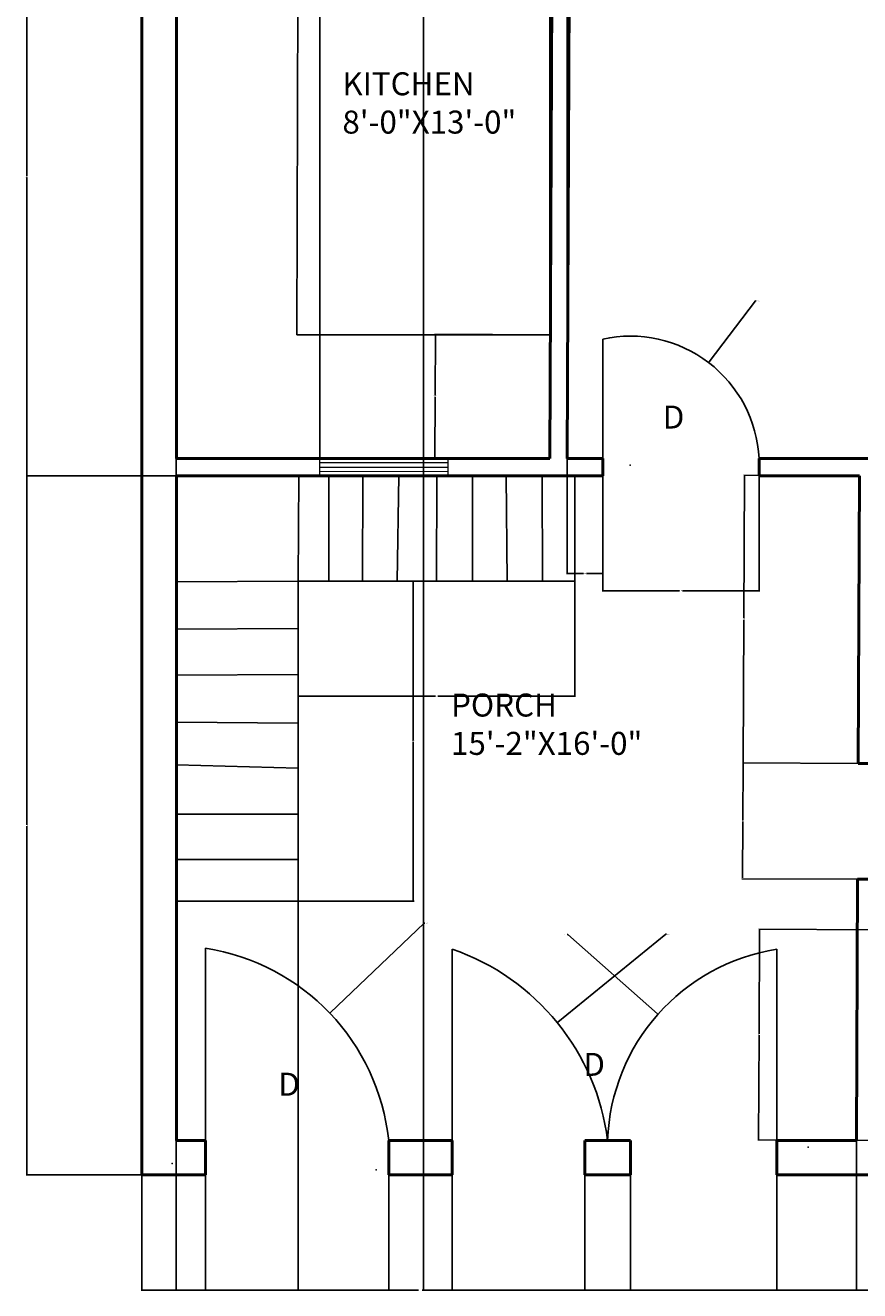
# Model space of a CAD drawing. Units: inches. Extents: x 2341 to 2761, y 2129 to 2789.
# Tile 1 of 4: x 2341 to 2559, y 2129 to 2459. Entities that reach past the tile are written whole.
import ezdxf

# ---------------------------------------------------------------- set-up
doc = ezdxf.new("R2010")
doc.units = ezdxf.units.IN
for name, color, linetype, lineweight in [('A-ANNO-DIMS', 2, 'Continuous', 18), ('A-ANNO-TEXT', 7, 'Continuous', 18), ('A-AREA-IDEN', 7, 'Continuous', 25), ('A-DOOR', 3, 'Continuous', 25), ('A-FLOR-FIXT', 9, 'Continuous', 25), ('A-FLOR-STRS', 7, 'Continuous', 25), ('A-GLAZ', 4, 'Continuous', 18), ('A-WALL', 7, 'Continuous', 50)]:
    doc.layers.add(name, color=color, linetype=linetype, lineweight=lineweight)
doc.styles.get("Standard").update_dxf_attribs({"font": 'arial.ttf'})
doc.dimstyles.get("Standard").update_dxf_attribs({"dimtxt": 0.18, "dimasz": 0.18, "dimexe": 0.18, "dimexo": 0.0625, "dimgap": 0.09, "dimtad": 0, "dimtih": 1, "dimtoh": 1, "dimdec": 4, "dimzin": 0, "dimdsep": 46, "dimtxsty": 'Standard', "dimcen": 0.09, "dimadec": 0, "dimazin": 0, "dimtfac": 1, "dimtdec": 4, "dimtofl": 0, "dimtmove": 0, "dimatfit": 3, "dimfxl": 1, "dimtolj": 1, "dimtzin": 0, "dimarcsym": 0})

# ---------------------------------------------------------------- blocks, each defined once
blk = doc.blocks.new('WIN-33IN-NARROW')
for p, q in [((0, 3.43), (33.34, 3.43)), ((0, 2.27), (33.34, 2.27)), ((0, 1.23), (33.34, 1.12))]:
    blk.add_line(p, q)
blk.add_lwpolyline([(0, 4.54), (33.34, 4.54), (33.34, 0), (0, 0)], close=True)
blk = doc.blocks.new('*D13')
at = {"layer": 'A-ANNO-DIMS', "color": 0, "lineweight": -2, "transparency": 16777216}
for p, q in [((2380.18, 2341.58), (2341.01, 2341.58)), ((2341.19, 2341.4), (2341.19, 2250.53)), ((2341.19, 2159.3), (2341.19, 2250.17)), ((2371.18, 2159.12), (2341.01, 2159.12))]:
    blk.add_line(p, q, dxfattribs=at)
at = {"layer": 'A-ANNO-DIMS', "color": 0, "transparency": 16777216}
for points in [[(2341.16, 2341.4), (2341.22, 2341.4), (2341.19, 2341.58)], [(2341.16, 2159.3), (2341.22, 2159.3), (2341.19, 2159.12)]]:
    blk.add_solid(points, dxfattribs=at)
at = {"layer": 'Defpoints', "color": 0, "transparency": 16777216}
for p in [(2341.19, 2341.58), (2380.24, 2341.58), (2371.24, 2159.12)]:
    blk.add_point(p, dxfattribs=at)
at = {"layer": 'A-ANNO-DIMS', "color": 0, "transparency": 16777216, "insert": (2341.19, 2250.35), "char_height": 0.18, "attachment_point": 5}
blk.add_mtext('\\A1;182.46', dxfattribs=at)
blk = doc.blocks.new('*D14')
at = {"layer": 'A-ANNO-DIMS', "color": 0, "lineweight": -2, "transparency": 16777216}
for p, q in [((2380.18, 2497.6), (2341.01, 2497.6)), ((2341.19, 2497.42), (2341.19, 2419.77)), ((2341.19, 2341.76), (2341.19, 2419.4)), ((2380.18, 2341.58), (2341.01, 2341.58))]:
    blk.add_line(p, q, dxfattribs=at)
at = {"layer": 'A-ANNO-DIMS', "color": 0, "transparency": 16777216}
for points in [[(2341.16, 2497.42), (2341.22, 2497.42), (2341.19, 2497.6)], [(2341.16, 2341.76), (2341.22, 2341.76), (2341.19, 2341.58)]]:
    blk.add_solid(points, dxfattribs=at)
at = {"layer": 'Defpoints', "color": 0, "transparency": 16777216}
for p in [(2341.19, 2497.6), (2380.24, 2497.6), (2380.24, 2341.58)]:
    blk.add_point(p, dxfattribs=at)
at = {"layer": 'A-ANNO-DIMS', "color": 0, "transparency": 16777216, "insert": (2341.19, 2419.59), "char_height": 0.18, "attachment_point": 5}
blk.add_mtext('\\A1;156.02', dxfattribs=at)
blk = doc.blocks.new('*D17')
at = {"layer": 'A-ANNO-DIMS', "color": 0, "lineweight": -2, "transparency": 16777216}
for p, q in [((2444.74, 2750.05), (2444.74, 2128.92)), ((2658.39, 2749.97), (2658.39, 2128.92)), ((2444.92, 2129.1), (2551.1, 2129.1)), ((2658.21, 2129.1), (2552.03, 2129.1))]:
    blk.add_line(p, q, dxfattribs=at)
at = {"layer": 'A-ANNO-DIMS', "color": 0, "transparency": 16777216}
for points in [[(2444.92, 2129.13), (2444.92, 2129.07), (2444.74, 2129.1)], [(2658.21, 2129.13), (2658.21, 2129.07), (2658.39, 2129.1)]]:
    blk.add_solid(points, dxfattribs=at)
at = {"layer": 'Defpoints', "color": 0, "transparency": 16777216}
for p in [(2444.74, 2750.12), (2658.39, 2750.04), (2658.39, 2129.1)]:
    blk.add_point(p, dxfattribs=at)
at = {"layer": 'A-ANNO-DIMS', "color": 0, "transparency": 16777216, "insert": (2551.56, 2129.1), "char_height": 0.18, "attachment_point": 5}
blk.add_mtext('\\A1;213.65', dxfattribs=at)
blk = doc.blocks.new('*D18')
at = {"layer": 'A-ANNO-DIMS', "color": 0, "lineweight": -2, "transparency": 16777216}
for p, q in [((2371.24, 2159.06), (2371.24, 2128.92)), ((2387.84, 2159.06), (2387.84, 2128.92)), ((2371.42, 2129.1), (2379.08, 2129.1)), ((2387.66, 2129.1), (2379.99, 2129.1))]:
    blk.add_line(p, q, dxfattribs=at)
at = {"layer": 'A-ANNO-DIMS', "color": 0, "transparency": 16777216}
for points in [[(2371.42, 2129.13), (2371.42, 2129.07), (2371.24, 2129.1)], [(2387.66, 2129.13), (2387.66, 2129.07), (2387.84, 2129.1)]]:
    blk.add_solid(points, dxfattribs=at)
at = {"layer": 'Defpoints', "color": 0, "transparency": 16777216}
for p in [(2371.24, 2159.12), (2387.84, 2159.12), (2387.84, 2129.1)]:
    blk.add_point(p, dxfattribs=at)
at = {"layer": 'A-ANNO-DIMS', "color": 0, "transparency": 16777216, "insert": (2379.54, 2129.1), "char_height": 0.18, "attachment_point": 5}
blk.add_mtext('\\A1;16.594', dxfattribs=at)
blk = doc.blocks.new('*D19')
at = {"layer": 'A-ANNO-DIMS', "color": 0, "lineweight": -2, "transparency": 16777216}
for p, q in [((2387.84, 2159.06), (2387.84, 2128.92)), ((2435.67, 2159.06), (2435.67, 2128.92)), ((2388.02, 2129.1), (2411.35, 2129.1)), ((2435.49, 2129.1), (2412.15, 2129.1))]:
    blk.add_line(p, q, dxfattribs=at)
at = {"layer": 'A-ANNO-DIMS', "color": 0, "transparency": 16777216}
for points in [[(2388.02, 2129.13), (2388.02, 2129.07), (2387.84, 2129.1)], [(2435.49, 2129.13), (2435.49, 2129.07), (2435.67, 2129.1)]]:
    blk.add_solid(points, dxfattribs=at)
at = {"layer": 'Defpoints', "color": 0, "transparency": 16777216}
for p in [(2387.84, 2159.12), (2435.67, 2159.12), (2435.67, 2129.1)]:
    blk.add_point(p, dxfattribs=at)
at = {"layer": 'A-ANNO-DIMS', "color": 0, "transparency": 16777216, "insert": (2411.75, 2129.1), "char_height": 0.18, "attachment_point": 5}
blk.add_mtext('\\A1;47.83', dxfattribs=at)
blk = doc.blocks.new('*D20')
at = {"layer": 'A-ANNO-DIMS', "color": 0, "lineweight": -2, "transparency": 16777216}
for p, q in [((2435.67, 2159.06), (2435.67, 2128.92)), ((2452.23, 2159.06), (2452.23, 2128.92)), ((2435.85, 2129.1), (2443.49, 2129.1)), ((2452.05, 2129.1), (2444.4, 2129.1))]:
    blk.add_line(p, q, dxfattribs=at)
at = {"layer": 'A-ANNO-DIMS', "color": 0, "transparency": 16777216}
for points in [[(2435.85, 2129.13), (2435.85, 2129.07), (2435.67, 2129.1)], [(2452.05, 2129.13), (2452.05, 2129.07), (2452.23, 2129.1)]]:
    blk.add_solid(points, dxfattribs=at)
at = {"layer": 'Defpoints', "color": 0, "transparency": 16777216}
for p in [(2435.67, 2159.12), (2452.23, 2159.12), (2452.23, 2129.1)]:
    blk.add_point(p, dxfattribs=at)
at = {"layer": 'A-ANNO-DIMS', "color": 0, "transparency": 16777216, "insert": (2443.95, 2129.1), "char_height": 0.18, "attachment_point": 5}
blk.add_mtext('\\A1;16.563', dxfattribs=at)
blk = doc.blocks.new('*D21')
at = {"layer": 'A-ANNO-DIMS', "color": 0, "lineweight": -2, "transparency": 16777216}
for p, q in [((2452.23, 2159.06), (2452.23, 2128.92)), ((2486.83, 2159.06), (2486.83, 2128.92)), ((2452.41, 2129.1), (2469.21, 2129.1)), ((2486.65, 2129.1), (2469.85, 2129.1))]:
    blk.add_line(p, q, dxfattribs=at)
at = {"layer": 'A-ANNO-DIMS', "color": 0, "transparency": 16777216}
for points in [[(2452.41, 2129.13), (2452.41, 2129.07), (2452.23, 2129.1)], [(2486.65, 2129.13), (2486.65, 2129.07), (2486.83, 2129.1)]]:
    blk.add_solid(points, dxfattribs=at)
at = {"layer": 'Defpoints', "color": 0, "transparency": 16777216}
for p in [(2452.23, 2159.12), (2486.83, 2159.12), (2486.83, 2129.1)]:
    blk.add_point(p, dxfattribs=at)
at = {"layer": 'A-ANNO-DIMS', "color": 0, "transparency": 16777216, "insert": (2469.53, 2129.1), "char_height": 0.18, "attachment_point": 5}
blk.add_mtext('\\A1;34.6', dxfattribs=at)
blk = doc.blocks.new('*D22')
at = {"layer": 'A-ANNO-DIMS', "color": 0, "lineweight": -2, "transparency": 16777216}
for p, q in [((2486.83, 2159.06), (2486.83, 2128.92)), ((2498.83, 2159.06), (2498.83, 2128.92)), ((2487.01, 2129.1), (2492.37, 2129.1)), ((2498.65, 2129.1), (2493.28, 2129.1))]:
    blk.add_line(p, q, dxfattribs=at)
at = {"layer": 'A-ANNO-DIMS', "color": 0, "transparency": 16777216}
for points in [[(2487.01, 2129.13), (2487.01, 2129.07), (2486.83, 2129.1)], [(2498.65, 2129.13), (2498.65, 2129.07), (2498.83, 2129.1)]]:
    blk.add_solid(points, dxfattribs=at)
at = {"layer": 'Defpoints', "color": 0, "transparency": 16777216}
for p in [(2486.83, 2159.12), (2498.83, 2159.12), (2498.83, 2129.1)]:
    blk.add_point(p, dxfattribs=at)
at = {"layer": 'A-ANNO-DIMS', "color": 0, "transparency": 16777216, "insert": (2492.83, 2129.1), "char_height": 0.18, "attachment_point": 5}
blk.add_mtext('\\A1;11.996', dxfattribs=at)
blk = doc.blocks.new('*D23')
at = {"layer": 'A-ANNO-DIMS', "color": 0, "lineweight": -2, "transparency": 16777216}
for p, q in [((2498.83, 2159.06), (2498.83, 2128.92)), ((2537.01, 2159.06), (2537.01, 2128.92)), ((2499.01, 2129.1), (2517.52, 2129.1)), ((2536.83, 2129.1), (2518.31, 2129.1))]:
    blk.add_line(p, q, dxfattribs=at)
at = {"layer": 'A-ANNO-DIMS', "color": 0, "transparency": 16777216}
for points in [[(2499.01, 2129.13), (2499.01, 2129.07), (2498.83, 2129.1)], [(2536.83, 2129.13), (2536.83, 2129.07), (2537.01, 2129.1)]]:
    blk.add_solid(points, dxfattribs=at)
at = {"layer": 'Defpoints', "color": 0, "transparency": 16777216}
for p in [(2498.83, 2159.12), (2537.01, 2159.12), (2537.01, 2129.1)]:
    blk.add_point(p, dxfattribs=at)
at = {"layer": 'A-ANNO-DIMS', "color": 0, "transparency": 16777216, "insert": (2517.92, 2129.1), "char_height": 0.18, "attachment_point": 5}
blk.add_mtext('\\A1;38.18', dxfattribs=at)
blk = doc.blocks.new('*D24')
at = {"layer": 'A-ANNO-DIMS', "color": 0, "lineweight": -2, "transparency": 16777216}
for p, q in [((2557.74, 2168.07), (2557.74, 2128.92)), ((2537.01, 2159.06), (2537.01, 2128.92)), ((2537.19, 2129.1), (2546.91, 2129.1)), ((2557.56, 2129.1), (2547.84, 2129.1))]:
    blk.add_line(p, q, dxfattribs=at)
at = {"layer": 'A-ANNO-DIMS', "color": 0, "transparency": 16777216}
for points in [[(2537.19, 2129.13), (2537.19, 2129.07), (2537.01, 2129.1)], [(2557.56, 2129.13), (2557.56, 2129.07), (2557.74, 2129.1)]]:
    blk.add_solid(points, dxfattribs=at)
at = {"layer": 'Defpoints', "color": 0, "transparency": 16777216}
for p in [(2557.74, 2168.13), (2537.01, 2159.12), (2557.74, 2129.1)]:
    blk.add_point(p, dxfattribs=at)
at = {"layer": 'A-ANNO-DIMS', "color": 0, "transparency": 16777216, "insert": (2547.37, 2129.1), "char_height": 0.18, "attachment_point": 5}
blk.add_mtext('\\A1;20.736', dxfattribs=at)
blk = doc.blocks.new('*D25')
at = {"layer": 'A-ANNO-DIMS', "color": 0, "lineweight": -2, "transparency": 16777216}
for p, q in [((2557.74, 2168.07), (2557.74, 2128.92)), ((2650.24, 2168.1), (2650.24, 2128.92)), ((2557.92, 2129.1), (2603.67, 2129.1)), ((2650.06, 2129.1), (2604.32, 2129.1))]:
    blk.add_line(p, q, dxfattribs=at)
at = {"layer": 'A-ANNO-DIMS', "color": 0, "transparency": 16777216}
for points in [[(2557.92, 2129.13), (2557.92, 2129.07), (2557.74, 2129.1)], [(2650.06, 2129.13), (2650.06, 2129.07), (2650.24, 2129.1)]]:
    blk.add_solid(points, dxfattribs=at)
at = {"layer": 'Defpoints', "color": 0, "transparency": 16777216}
for p in [(2557.74, 2168.13), (2650.24, 2168.16), (2650.24, 2129.1)]:
    blk.add_point(p, dxfattribs=at)
at = {"layer": 'A-ANNO-DIMS', "color": 0, "transparency": 16777216, "insert": (2603.99, 2129.1), "char_height": 0.18, "attachment_point": 5}
blk.add_mtext('\\A1;92.5', dxfattribs=at)
blk = doc.blocks.new('*D27')
at = {"layer": 'A-ANNO-DIMS', "color": 0, "lineweight": -2, "transparency": 16777216}
for p, q in [((2380.24, 2230.49), (2380.24, 2128.92)), ((2412.08, 2230.49), (2412.08, 2128.92)), ((2380.42, 2129.1), (2395.77, 2129.1)), ((2411.9, 2129.1), (2396.56, 2129.1))]:
    blk.add_line(p, q, dxfattribs=at)
at = {"layer": 'A-ANNO-DIMS', "color": 0, "transparency": 16777216}
for points in [[(2380.42, 2129.13), (2380.42, 2129.07), (2380.24, 2129.1)], [(2411.9, 2129.13), (2411.9, 2129.07), (2412.08, 2129.1)]]:
    blk.add_solid(points, dxfattribs=at)
at = {"layer": 'Defpoints', "color": 0, "transparency": 16777216}
for p in [(2380.24, 2230.56), (2412.08, 2230.56), (2412.08, 2129.1)]:
    blk.add_point(p, dxfattribs=at)
at = {"layer": 'A-ANNO-DIMS', "color": 0, "transparency": 16777216, "insert": (2396.16, 2129.1), "char_height": 0.18, "attachment_point": 5}
blk.add_mtext('\\A1;31.84', dxfattribs=at)
blk = doc.blocks.new('*D28')
at = {"layer": 'A-ANNO-DIMS', "color": 0, "lineweight": -2, "transparency": 16777216}
for p, q in [((2477.74, 2346.18), (2477.74, 2789.36)), ((2477.92, 2789.18), (2479.73, 2789.18)), ((2482.06, 2789.18), (2480.25, 2789.18)), ((2482.24, 2346.16), (2482.24, 2789.36))]:
    blk.add_line(p, q, dxfattribs=at)
at = {"layer": 'A-ANNO-DIMS', "color": 0, "transparency": 16777216}
for points in [[(2477.92, 2789.21), (2477.92, 2789.15), (2477.74, 2789.18)], [(2482.06, 2789.21), (2482.06, 2789.15), (2482.24, 2789.18)]]:
    blk.add_solid(points, dxfattribs=at)
at = {"layer": 'Defpoints', "color": 0, "transparency": 16777216}
for p in [(2482.24, 2789.18), (2477.74, 2346.12), (2482.24, 2346.1)]:
    blk.add_point(p, dxfattribs=at)
at = {"layer": 'A-ANNO-DIMS', "color": 0, "transparency": 16777216, "insert": (2479.99, 2789.18), "char_height": 0.18, "attachment_point": 5}
blk.add_mtext('\\A1;4.5', dxfattribs=at)
blk = doc.blocks.new('*D29')
at = {"layer": 'A-ANNO-DIMS', "color": 0, "lineweight": -2, "transparency": 16777216}
for p, q in [((2371.24, 2759.06), (2371.24, 2128.92)), ((2380.24, 2750.06), (2380.24, 2128.92)), ((2371.42, 2129.1), (2375.59, 2129.1)), ((2380.06, 2129.1), (2375.89, 2129.1))]:
    blk.add_line(p, q, dxfattribs=at)
at = {"layer": 'A-ANNO-DIMS', "color": 0, "transparency": 16777216}
for points in [[(2371.42, 2129.13), (2371.42, 2129.07), (2371.24, 2129.1)], [(2380.06, 2129.13), (2380.06, 2129.07), (2380.24, 2129.1)]]:
    blk.add_solid(points, dxfattribs=at)
at = {"layer": 'Defpoints', "color": 0, "transparency": 16777216}
for p in [(2371.24, 2759.12), (2380.24, 2750.12), (2380.24, 2129.1)]:
    blk.add_point(p, dxfattribs=at)
at = {"layer": 'A-ANNO-DIMS', "color": 0, "transparency": 16777216, "insert": (2375.74, 2129.1), "char_height": 0.18, "attachment_point": 5}
blk.add_mtext('\\A1;9', dxfattribs=at)
blk = doc.blocks.new('*D30')
at = {"layer": 'A-ANNO-DIMS', "color": 0, "lineweight": -2, "transparency": 16777216}
for p, q in [((2562.45, 2223.1), (2532.31, 2223.25)), ((2532.49, 2223.06), (2532.36, 2195.94)), ((2532.22, 2168.45), (2532.36, 2195.58)), ((2562.18, 2168.12), (2532.04, 2168.27))]:
    blk.add_line(p, q, dxfattribs=at)
at = {"layer": 'A-ANNO-DIMS', "color": 0, "transparency": 16777216}
for points in [[(2532.46, 2223.06), (2532.52, 2223.06), (2532.49, 2223.24)], [(2532.19, 2168.45), (2532.25, 2168.45), (2532.22, 2168.27)]]:
    blk.add_solid(points, dxfattribs=at)
at = {"layer": 'Defpoints', "color": 0, "transparency": 16777216}
for p in [(2532.49, 2223.24), (2562.51, 2223.1), (2562.24, 2168.12)]:
    blk.add_point(p, dxfattribs=at)
at = {"layer": 'A-ANNO-DIMS', "color": 0, "transparency": 16777216, "insert": (2532.36, 2195.76), "char_height": 0.18, "attachment_point": 5}
blk.add_mtext('\\A1;54.97', dxfattribs=at)
blk = doc.blocks.new('*D33')
at = {"layer": 'A-ANNO-DIMS', "color": 0, "lineweight": -2, "transparency": 16777216}
for p, q in [((2380.24, 2346.14), (2380.24, 2789.36)), ((2380.42, 2789.18), (2398.59, 2789.18)), ((2417.55, 2789.18), (2399.38, 2789.18)), ((2417.73, 2346.19), (2417.73, 2789.36))]:
    blk.add_line(p, q, dxfattribs=at)
at = {"layer": 'A-ANNO-DIMS', "color": 0, "transparency": 16777216}
for points in [[(2380.42, 2789.21), (2380.42, 2789.15), (2380.24, 2789.18)], [(2417.55, 2789.21), (2417.55, 2789.15), (2417.73, 2789.18)]]:
    blk.add_solid(points, dxfattribs=at)
at = {"layer": 'Defpoints', "color": 0, "transparency": 16777216}
for p in [(2417.73, 2789.18), (2380.24, 2346.08), (2417.73, 2346.13)]:
    blk.add_point(p, dxfattribs=at)
at = {"layer": 'A-ANNO-DIMS', "color": 0, "transparency": 16777216, "insert": (2398.99, 2789.18), "char_height": 0.18, "attachment_point": 5}
blk.add_mtext('\\A1;37.49', dxfattribs=at)
blk = doc.blocks.new('*D49')
at = {"layer": 'A-ANNO-DIMS', "color": 0, "lineweight": -2, "transparency": 16777216}
for p, q in [((2482.24, 2346.03), (2482.24, 2315.9)), ((2491.53, 2346.03), (2491.53, 2315.9)), ((2482.42, 2316.08), (2486.49, 2316.08)), ((2491.35, 2316.08), (2487.28, 2316.08))]:
    blk.add_line(p, q, dxfattribs=at)
at = {"layer": 'A-ANNO-DIMS', "color": 0, "transparency": 16777216}
for points in [[(2482.42, 2316.11), (2482.42, 2316.05), (2482.24, 2316.08)], [(2491.35, 2316.11), (2491.35, 2316.05), (2491.53, 2316.08)]]:
    blk.add_solid(points, dxfattribs=at)
at = {"layer": 'Defpoints', "color": 0, "transparency": 16777216}
for p in [(2482.24, 2346.1), (2491.53, 2346.1), (2482.24, 2316.08)]:
    blk.add_point(p, dxfattribs=at)
at = {"layer": 'A-ANNO-DIMS', "color": 0, "transparency": 16777216, "insert": (2486.89, 2316.08), "char_height": 0.18, "attachment_point": 5}
blk.add_mtext('\\A1;9.296', dxfattribs=at)
blk = doc.blocks.new('*D50')
at = {"layer": 'A-ANNO-DIMS', "color": 0, "lineweight": -2, "transparency": 16777216}
for p, q in [((2491.53, 2341.53), (2491.53, 2311.4)), ((2532.36, 2341.53), (2532.36, 2311.4)), ((2491.71, 2311.58), (2511.55, 2311.58)), ((2532.18, 2311.58), (2512.34, 2311.58))]:
    blk.add_line(p, q, dxfattribs=at)
at = {"layer": 'A-ANNO-DIMS', "color": 0, "transparency": 16777216}
for points in [[(2491.71, 2311.61), (2491.71, 2311.55), (2491.53, 2311.58)], [(2532.18, 2311.61), (2532.18, 2311.55), (2532.36, 2311.58)]]:
    blk.add_solid(points, dxfattribs=at)
at = {"layer": 'Defpoints', "color": 0, "transparency": 16777216}
for p in [(2491.53, 2341.6), (2532.36, 2341.6), (2491.53, 2311.58)]:
    blk.add_point(p, dxfattribs=at)
at = {"layer": 'A-ANNO-DIMS', "color": 0, "transparency": 16777216, "insert": (2511.95, 2311.58), "char_height": 0.18, "attachment_point": 5}
blk.add_mtext('\\A1;40.82', dxfattribs=at)
blk = doc.blocks.new('*D51')
at = {"layer": 'A-ANNO-DIMS', "color": 0, "lineweight": -2, "transparency": 16777216}
for p, q in [((2558.17, 2266.54), (2528.03, 2266.69)), ((2528.21, 2266.51), (2528.14, 2251.75)), ((2528.06, 2236.62), (2528.13, 2251.38)), ((2558.02, 2236.29), (2527.88, 2236.44))]:
    blk.add_line(p, q, dxfattribs=at)
at = {"layer": 'A-ANNO-DIMS', "color": 0, "transparency": 16777216}
for points in [[(2528.18, 2266.51), (2528.24, 2266.51), (2528.21, 2266.69)], [(2528.03, 2236.62), (2528.09, 2236.62), (2528.06, 2236.44)]]:
    blk.add_solid(points, dxfattribs=at)
at = {"layer": 'Defpoints', "color": 0, "transparency": 16777216}
for p in [(2528.21, 2266.69), (2558.23, 2266.54), (2558.08, 2236.29)]:
    blk.add_point(p, dxfattribs=at)
at = {"layer": 'A-ANNO-DIMS', "color": 0, "transparency": 16777216, "insert": (2528.14, 2251.56), "char_height": 0.18, "attachment_point": 5}
blk.add_mtext('\\A1;30.25', dxfattribs=at)
blk = doc.blocks.new('*D52')
at = {"layer": 'A-ANNO-DIMS', "color": 0, "lineweight": -2, "transparency": 16777216}
for p, q in [((2558.54, 2341.6), (2528.4, 2341.75)), ((2528.58, 2341.56), (2528.4, 2304.4)), ((2528.21, 2266.87), (2528.4, 2304.03)), ((2558.17, 2266.54), (2528.03, 2266.69))]:
    blk.add_line(p, q, dxfattribs=at)
at = {"layer": 'A-ANNO-DIMS', "color": 0, "transparency": 16777216}
for points in [[(2528.55, 2341.56), (2528.61, 2341.56), (2528.58, 2341.74)], [(2528.18, 2266.87), (2528.24, 2266.87), (2528.21, 2266.69)]]:
    blk.add_solid(points, dxfattribs=at)
at = {"layer": 'Defpoints', "color": 0, "transparency": 16777216}
for p in [(2528.58, 2341.74), (2558.6, 2341.6), (2558.23, 2266.54)]:
    blk.add_point(p, dxfattribs=at)
at = {"layer": 'A-ANNO-DIMS', "color": 0, "transparency": 16777216, "insert": (2528.4, 2304.22), "char_height": 0.18, "attachment_point": 5}
blk.add_mtext('\\A1;75.06', dxfattribs=at)
blk = doc.blocks.new('*D56')
at = {"layer": 'A-ANNO-DIMS', "color": 0, "lineweight": -2, "transparency": 16777216}
for p, q in [((2412.15, 2314.12), (2442.28, 2314.12)), ((2442.1, 2313.94), (2442.1, 2272.52)), ((2442.1, 2230.74), (2442.1, 2272.16)), ((2412.15, 2230.56), (2442.28, 2230.56))]:
    blk.add_line(p, q, dxfattribs=at)
at = {"layer": 'A-ANNO-DIMS', "color": 0, "transparency": 16777216}
for points in [[(2442.07, 2313.94), (2442.13, 2313.94), (2442.1, 2314.12)], [(2442.07, 2230.74), (2442.13, 2230.74), (2442.1, 2230.56)]]:
    blk.add_solid(points, dxfattribs=at)
at = {"layer": 'Defpoints', "color": 0, "transparency": 16777216}
for p in [(2412.08, 2314.12), (2412.08, 2230.56), (2442.1, 2230.56)]:
    blk.add_point(p, dxfattribs=at)
at = {"layer": 'A-ANNO-DIMS', "color": 0, "transparency": 16777216, "insert": (2442.1, 2272.34), "char_height": 0.18, "attachment_point": 5}
blk.add_mtext('\\A1;83.57', dxfattribs=at)
blk = doc.blocks.new('*D57')
at = {"layer": 'A-ANNO-DIMS', "color": 0, "lineweight": -2, "transparency": 16777216}
for p, q in [((2412.08, 2314.06), (2412.08, 2283.92)), ((2484.28, 2314.06), (2484.28, 2283.92)), ((2412.26, 2284.1), (2447.86, 2284.1)), ((2484.1, 2284.1), (2448.5, 2284.1))]:
    blk.add_line(p, q, dxfattribs=at)
at = {"layer": 'A-ANNO-DIMS', "color": 0, "transparency": 16777216}
for points in [[(2412.26, 2284.13), (2412.26, 2284.07), (2412.08, 2284.1)], [(2484.1, 2284.13), (2484.1, 2284.07), (2484.28, 2284.1)]]:
    blk.add_solid(points, dxfattribs=at)
at = {"layer": 'Defpoints', "color": 0, "transparency": 16777216}
for p in [(2412.08, 2314.12), (2484.28, 2314.12), (2412.08, 2284.1)]:
    blk.add_point(p, dxfattribs=at)
at = {"layer": 'A-ANNO-DIMS', "color": 0, "transparency": 16777216, "insert": (2448.18, 2284.1), "char_height": 0.18, "attachment_point": 5}
blk.add_mtext('\\A1;72.2', dxfattribs=at)
blk = doc.blocks.new('*D59')
at = {"layer": 'A-ANNO-DIMS', "color": 0, "lineweight": -2, "transparency": 16777216}
for p, q in [((2477.82, 2378.38), (2447.68, 2378.51)), ((2447.86, 2378.33), (2447.79, 2362.56)), ((2447.72, 2346.43), (2447.79, 2362.2)), ((2477.68, 2346.12), (2447.54, 2346.25))]:
    blk.add_line(p, q, dxfattribs=at)
at = {"layer": 'A-ANNO-DIMS', "color": 0, "transparency": 16777216}
for points in [[(2447.83, 2378.33), (2447.89, 2378.33), (2447.86, 2378.51)], [(2447.69, 2346.43), (2447.75, 2346.43), (2447.72, 2346.25)]]:
    blk.add_solid(points, dxfattribs=at)
at = {"layer": 'Defpoints', "color": 0, "transparency": 16777216}
for p in [(2447.86, 2378.51), (2477.88, 2378.38), (2477.74, 2346.12)]:
    blk.add_point(p, dxfattribs=at)
at = {"layer": 'A-ANNO-DIMS', "color": 0, "transparency": 16777216, "insert": (2447.79, 2362.38), "char_height": 0.18, "attachment_point": 5}
blk.add_mtext('\\A1;32.265', dxfattribs=at)
blk = doc.blocks.new('*D62')
at = {"layer": 'A-ANNO-DIMS', "color": 0, "lineweight": -2, "transparency": 16777216}
for p, q in [((2508.03, 2221.95), (2479.79, 2199)), ((2508.21, 2221.95), (2508.03, 2221.95)), ((2432.28, 2160.44), (2432.46, 2160.44)), ((2432.37, 2160.35), (2432.37, 2160.53))]:
    blk.add_line(p, q, dxfattribs=at)
at = {"layer": 'A-ANNO-DIMS', "color": 0, "transparency": 16777216}
blk.add_solid([(2479.78, 2199.02), (2479.81, 2198.98), (2479.66, 2198.89)], dxfattribs=at)
at = {"layer": 'Defpoints', "color": 0, "transparency": 16777216}
for p in [(2479.66, 2198.89), (2432.37, 2160.44)]:
    blk.add_point(p, dxfattribs=at)
at = {"layer": 'A-ANNO-DIMS', "color": 0, "transparency": 16777216, "insert": (2508.69, 2221.95), "char_height": 0.18, "attachment_point": 5}
blk.add_mtext('\\A1;R60.94', dxfattribs=at)
blk = doc.blocks.new('*D63')
at = {"layer": 'A-ANNO-DIMS', "color": 0, "lineweight": -2, "transparency": 16777216}
for p, q in [((2444.95, 2224.86), (2420.42, 2201.47)), ((2445.13, 2224.86), (2444.95, 2224.86)), ((2379.1, 2162.15), (2379.28, 2162.15)), ((2379.19, 2162.06), (2379.19, 2162.24))]:
    blk.add_line(p, q, dxfattribs=at)
at = {"layer": 'A-ANNO-DIMS', "color": 0, "transparency": 16777216}
blk.add_solid([(2420.4, 2201.49), (2420.44, 2201.45), (2420.29, 2201.34)], dxfattribs=at)
at = {"layer": 'Defpoints', "color": 0, "transparency": 16777216}
for p in [(2420.29, 2201.34), (2379.19, 2162.15)]:
    blk.add_point(p, dxfattribs=at)
at = {"layer": 'A-ANNO-DIMS', "color": 0, "transparency": 16777216, "insert": (2445.61, 2224.86), "char_height": 0.18, "attachment_point": 5}
blk.add_mtext('\\A1;R56.79', dxfattribs=at)
blk = doc.blocks.new('*D64')
at = {"layer": 'A-ANNO-DIMS', "color": 0, "lineweight": -2, "transparency": 16777216}
for p, q in [((2482.24, 2221.84), (2482.42, 2221.84)), ((2482.42, 2221.84), (2505.8, 2201.16)), ((2545.04, 2166.36), (2545.22, 2166.36)), ((2545.13, 2166.27), (2545.13, 2166.45))]:
    blk.add_line(p, q, dxfattribs=at)
at = {"layer": 'A-ANNO-DIMS', "color": 0, "transparency": 16777216}
blk.add_solid([(2505.82, 2201.18), (2505.78, 2201.13), (2505.94, 2201.04)], dxfattribs=at)
at = {"layer": 'Defpoints', "color": 0, "transparency": 16777216}
for p in [(2505.94, 2201.04), (2545.13, 2166.36)]:
    blk.add_point(p, dxfattribs=at)
at = {"layer": 'A-ANNO-DIMS', "color": 0, "transparency": 16777216, "insert": (2481.76, 2221.84), "char_height": 0.18, "attachment_point": 5}
blk.add_mtext('\\A1;R52.33', dxfattribs=at)
blk = doc.blocks.new('*D70')
at = {"layer": 'A-ANNO-DIMS', "color": 0, "lineweight": -2, "transparency": 16777216}
for p, q in [((2531.43, 2387.2), (2519.28, 2371.28)), ((2531.61, 2387.2), (2531.43, 2387.2)), ((2498.63, 2344.38), (2498.81, 2344.38)), ((2498.72, 2344.29), (2498.72, 2344.47))]:
    blk.add_line(p, q, dxfattribs=at)
at = {"layer": 'A-ANNO-DIMS', "color": 0, "transparency": 16777216}
blk.add_solid([(2519.25, 2371.3), (2519.3, 2371.26), (2519.17, 2371.14)], dxfattribs=at)
at = {"layer": 'Defpoints', "color": 0, "transparency": 16777216}
for p in [(2519.17, 2371.14), (2498.72, 2344.38)]:
    blk.add_point(p, dxfattribs=at)
at = {"layer": 'A-ANNO-DIMS', "color": 0, "transparency": 16777216, "insert": (2532.16, 2387.2), "char_height": 0.18, "attachment_point": 5}
blk.add_mtext('\\A1;R33.677', dxfattribs=at)

msp = doc.modelspace()

# ---------------------------------------------------------------- linework, layer by layer
at = {"layer": 'A-DOOR'}
for p, q in [((2491.5341, 2346.0958), (2491.5341, 2377.2773)), ((2387.8363, 2168.1222), (2387.8363, 2218.2792)), ((2452.2283, 2168.1247), (2452.2283, 2218.0539)), ((2537.0059, 2168.128), (2537.0057, 2218.0539))]:
    msp.add_line(p, q, dxfattribs=at)
for centre, radius, start, end in [((2498.7241, 2344.3772), 33.6765, 2.925153, 102.327529), ((2379.1921, 2162.1527), 56.7882, 6.035859, 81.244458), ((2432.3705, 2160.4354), 60.9444, 7.249744, 70.983867), ((2545.1263, 2166.3593), 52.3286, 98.927508, 178.064871)]:
    msp.add_arc(centre, radius, start, end, dxfattribs=at)
at = {"layer": 'A-FLOR-FIXT'}
for p, q in [((2411.7316, 2378.3809), (2412.0874, 2497.5958)), ((2477.8811, 2378.3809), (2411.7316, 2378.3809))]:
    msp.add_line(p, q, dxfattribs=at)
at = {"layer": 'A-FLOR-STRS'}
for p, q in [((2412.0845, 2314.1234), (2412.2571, 2341.5831)), ((2420.0237, 2314.1234), (2420.0236, 2341.5845)), ((2428.8188, 2314.1234), (2428.9607, 2341.5861)), ((2437.8824, 2314.1234), (2438.3072, 2341.5878)), ((2448.1827, 2314.1234), (2448.2205, 2341.5896)), ((2457.5672, 2314.1234), (2457.5672, 2341.5913)), ((2466.6307, 2314.1234), (2466.3475, 2341.5929)), ((2475.8359, 2314.1234), (2475.6942, 2341.5946)), ((2484.281, 2314.1234), (2484.281, 2341.5958)), ((2412.0845, 2314.1234), (2380.242, 2313.8851)), ((2412.0845, 2230.5563), (2412.0845, 2314.1234)), ((2412.0845, 2314.1234), (2484.281, 2314.1234)), ((2412.0845, 2301.7549), (2380.242, 2301.5284)), ((2412.0845, 2289.7474), (2380.242, 2289.5209)), ((2412.0845, 2277.0603), (2380.242, 2277.2869)), ((2412.0845, 2265.2794), (2380.242, 2266.1856)), ((2412.0845, 2253.2719), (2380.242, 2253.2719)), ((2412.0845, 2241.491), (2380.242, 2241.491)), ((2380.242, 2230.5563), (2412.0845, 2230.5563))]:
    msp.add_line(p, q, dxfattribs=at)
at = {"layer": 'A-WALL'}
for p, q in [((2371.242, 2159.1219), (2371.242, 2759.1219)), ((2380.242, 2346.0773), (2380.242, 2497.5958)), ((2477.7379, 2346.1158), (2478.3031, 2473.4534)), ((2482.2379, 2346.0958), (2482.8032, 2473.4534)), ((2380.242, 2346.0773), (2477.7379, 2346.1158)), ((2491.5341, 2346.0958), (2482.2379, 2346.0958)), ((2491.5341, 2346.0958), (2491.5341, 2341.5958)), ((2722.2379, 2346.0958), (2532.3567, 2346.0958)), ((2532.3567, 2346.0958), (2532.3567, 2341.5958)), ((2482.2387, 2341.5958), (2380.242, 2341.5773)), ((2380.242, 2168.1219), (2380.242, 2341.5773)), ((2491.5341, 2341.5958), (2482.2379, 2341.5958)), ((2558.6015, 2341.5958), (2532.3567, 2341.5958)), ((2558.2296, 2266.54), (2558.6015, 2341.5958)), ((2558.2296, 2266.54), (2562.7297, 2266.54)), ((2557.7421, 2168.1288), (2558.0798, 2236.2899)), ((2558.0798, 2236.2899), (2562.5798, 2236.2899)), ((2380.242, 2168.1219), (2387.8363, 2168.1222)), ((2387.8363, 2168.1222), (2387.8363, 2159.1219)), ((2435.6655, 2168.1241), (2452.2283, 2168.1247)), ((2435.6655, 2168.1241), (2435.6655, 2159.1219)), ((2452.2283, 2168.1247), (2452.2283, 2159.1219)), ((2486.8294, 2168.1261), (2498.8259, 2168.1265)), ((2486.8294, 2168.1261), (2486.8294, 2159.1219)), ((2498.8259, 2168.1265), (2498.8259, 2159.1219)), ((2537.0059, 2168.128), (2557.7421, 2168.1288)), ((2537.0059, 2168.128), (2537.006, 2159.1219)), ((2387.8363, 2159.1219), (2371.242, 2159.1219)), ((2452.2283, 2159.1219), (2435.6655, 2159.1219)), ((2498.8259, 2159.1219), (2486.8294, 2159.1219)), ((2731.242, 2159.1219), (2537.006, 2159.1219))]:
    msp.add_line(p, q, dxfattribs=at)

# ---------------------------------------------------------------- block references
at = {"layer": 'A-GLAZ'}
msp.add_blockref('WIN-33IN-NARROW', (2417.7311, 2341.5842), dxfattribs=at)

# ---------------------------------------------------------------- texts
at = {"layer": 'A-ANNO-TEXT', "char_height": 6, "attachment_point": 1}
for insert in [(2507.2133, 2359.9074), (2486.4801, 2190.9776), (2406.8635, 2185.8064)]:
    msp.add_mtext_dynamic_manual_height_columns('D', width=9.002909, gutter_width=12.5, heights=[0], dxfattribs=dict(at, insert=insert))
at = {"layer": 'A-AREA-IDEN', "char_height": 6, "attachment_point": 1}
for s, width, insert in [('KITCHEN \\P8\'-0"X13\'-0"', 36.809608, (2423.5911, 2446.8818)), ('PORCH\\P15\'-2"X16\'-0"', 72.299204, (2451.9445, 2284.7541))]:
    msp.add_mtext_dynamic_manual_height_columns(s, width=width, gutter_width=12.5, heights=[0], dxfattribs=dict(at, insert=insert))

# ---------------------------------------------------------------- dimensions: what is measured, and where the dimension line sits
at = {"layer": 'A-ANNO-DIMS'}
for base, p1, p2, override, picture, middle in [((2417.7307, 2789.1821), (2380.242, 2346.0773), (2417.7307, 2346.1252), {"dimdec": 2, "dimlfac": 1, "dimrnd": 0, "dimzin": 0, "dimdsep": 46, "dimlunit": 2}, '*D33', (2398.9864, 2789.1821)), ((2482.2379, 2789.1821), (2477.7379, 2346.1158), (2482.2379, 2346.0958), {"dimdec": 1, "dimlfac": 1, "dimrnd": 0, "dimzin": 0, "dimdsep": 46, "dimlunit": 2}, '*D28', (2479.9879, 2789.1821)), ((2380.242, 2129.1019), (2371.242, 2759.1219), (2380.242, 2750.1219), {"dimdec": 0, "dimlfac": 1, "dimrnd": 0, "dimzin": 0, "dimdsep": 46, "dimlunit": 2}, '*D29', (2375.742, 2129.1019)), ((2658.3873, 2129.1019), (2444.742, 2750.1173), (2658.3873, 2750.0366), {"dimdec": 2, "dimlfac": 1, "dimrnd": 0, "dimzin": 0, "dimdsep": 46, "dimlunit": 2}, '*D17', (2551.5646, 2129.1019)), ((2412.0845, 2129.1019), (2380.242, 2230.5563), (2412.0845, 2230.5563), {"dimdec": 2, "dimlfac": 1, "dimrnd": 0, "dimzin": 0, "dimdsep": 46, "dimlunit": 2}, '*D27', (2396.1633, 2129.1019)), ((2557.7421, 2129.1019), (2537.006, 2159.1219), (2557.7421, 2168.1288), {"dimdec": 3, "dimlfac": 1, "dimrnd": 0, "dimzin": 0, "dimdsep": 46, "dimlunit": 2}, '*D24', (2547.374, 2129.1019)), ((2650.2421, 2129.1019), (2557.7421, 2168.1288), (2650.2421, 2168.1606), {"dimdec": 1, "dimlfac": 1, "dimrnd": 0, "dimzin": 0, "dimdsep": 46, "dimlunit": 2}, '*D25', (2603.9921, 2129.1019)), ((2387.8363, 2129.1019), (2371.242, 2159.1219), (2387.8363, 2159.1219), {"dimdec": 3, "dimlfac": 1, "dimrnd": 0, "dimzin": 0, "dimdsep": 46, "dimlunit": 2}, '*D18', (2379.5392, 2129.1019)), ((2435.6655, 2129.1019), (2387.8363, 2159.1219), (2435.6655, 2159.1219), {"dimdec": 2, "dimlfac": 1, "dimrnd": 0, "dimzin": 0, "dimdsep": 46, "dimlunit": 2}, '*D19', (2411.7509, 2129.1019)), ((2452.2283, 2129.1019), (2435.6655, 2159.1219), (2452.2283, 2159.1219), {"dimdec": 3, "dimlfac": 1, "dimrnd": 0, "dimzin": 0, "dimdsep": 46, "dimlunit": 2}, '*D20', (2443.9469, 2129.1019)), ((2486.8294, 2129.1019), (2452.2283, 2159.1219), (2486.8294, 2159.1219), {"dimdec": 1, "dimlfac": 1, "dimrnd": 0, "dimzin": 0, "dimdsep": 46, "dimlunit": 2}, '*D21', (2469.5288, 2129.1019)), ((2498.82587, 2129.10189), (2486.82938, 2159.12189), (2498.82587, 2159.12189), {"dimdec": 3, "dimlfac": 1, "dimrnd": 0, "dimzin": 0, "dimdsep": 46, "dimlunit": 2}, '*D22', (2492.82763, 2129.10189)), ((2537.006, 2129.1019), (2498.8259, 2159.1219), (2537.006, 2159.1219), {"dimdec": 2, "dimlfac": 1, "dimrnd": 0, "dimzin": 0, "dimdsep": 46, "dimlunit": 2}, '*D23', (2517.9159, 2129.1019))]:
    dim = msp.add_linear_dim(base=base, p1=p1, p2=p2, dimstyle='Standard', override=override, dxfattribs=at)
    dim.commit()
    dim.dimension.update_dxf_attribs({"geometry": picture, "text_midpoint": middle})
for base, p1, p2, angle, override, picture, middle in [((2341.1943, 2497.5958), (2380.242, 2341.5773), (2380.242, 2497.5958), 90, {"dimdec": 2, "dimlfac": 1, "dimrnd": 0, "dimzin": 0, "dimdsep": 46, "dimlunit": 2}, '*D14', (2341.1943, 2419.5865)), ((2447.8614, 2378.5141), (2477.7379, 2346.1158), (2477.8811, 2378.3809), 89.745684, {"dimdec": 3, "dimlfac": 1, "dimrnd": 0, "dimzin": 0, "dimdsep": 46, "dimlunit": 2}, '*D59', (2447.7898, 2362.3816)), ((2482.2379, 2316.0758), (2491.5341, 2346.0958), (2482.2379, 2346.0958), 180, {"dimdec": 3, "dimlfac": 1, "dimrnd": 0, "dimzin": 0, "dimdsep": 46, "dimlunit": 2}, '*D49', (2486.886, 2316.0758)), ((2341.1943, 2341.5773), (2371.242, 2159.1219), (2380.242, 2341.5773), 90, {"dimdec": 2, "dimlfac": 1, "dimrnd": 0, "dimzin": 0, "dimdsep": 46, "dimlunit": 2}, '*D13', (2341.1943, 2250.3496)), ((2491.5341, 2311.5758), (2532.3567, 2341.5958), (2491.5341, 2341.5958), 180, {"dimdec": 2, "dimlfac": 1, "dimrnd": 0, "dimzin": 0, "dimdsep": 46, "dimlunit": 2}, '*D50', (2511.9454, 2311.5758)), ((2528.5818, 2341.7445), (2558.2296, 2266.54), (2558.6015, 2341.5958), 89.716153, {"dimdec": 2, "dimlfac": 1, "dimrnd": 0, "dimzin": 0, "dimdsep": 46, "dimlunit": 2}, '*D52', (2528.3959, 2304.2166)), ((2442.1045, 2230.5563), (2412.0845, 2314.1234), (2412.0845, 2230.5563), 270, {"dimdec": 2, "dimlfac": 1, "dimrnd": 0, "dimzin": 0, "dimdsep": 46, "dimlunit": 2}, '*D56', (2442.1045, 2272.3398)), ((2412.0845, 2284.1034), (2484.281, 2314.1234), (2412.0845, 2314.1234), 180, {"dimdec": 1, "dimlfac": 1, "dimrnd": 0, "dimzin": 0, "dimdsep": 46, "dimlunit": 2}, '*D57', (2448.1827, 2284.1034)), ((2528.21, 2266.6887), (2558.0798, 2236.2899), (2558.2296, 2266.54), 89.716153, {"dimdec": 2, "dimlfac": 1, "dimrnd": 0, "dimzin": 0, "dimdsep": 46, "dimlunit": 2}, '*D51', (2528.1351, 2251.5636)), ((2532.4948, 2223.2447), (2562.2421, 2168.1219), (2562.5145, 2223.096), 89.716153, {"dimdec": 2, "dimlfac": 1, "dimrnd": 0, "dimzin": 0, "dimdsep": 46, "dimlunit": 2}, '*D30', (2532.3587, 2195.7577))]:
    dim = msp.add_linear_dim(base=base, p1=p1, p2=p2, angle=angle, dimstyle='Standard', override=override, dxfattribs=at)
    dim.commit()
    dim.dimension.update_dxf_attribs({"geometry": picture, "text_midpoint": middle})
for center, mpoint, override, picture, middle in [((2498.7241, 2344.3772), (2519.1659, 2371.1399), {"dimdec": 3, "dimlfac": 1, "dimrnd": 0, "dimzin": 0, "dimdsep": 46, "dimlunit": 2}, '*D70', (2532.1608, 2387.1974)), ((2379.1921, 2162.1527), (2420.2889, 2201.3439), {"dimdec": 2, "dimlfac": 1, "dimrnd": 0, "dimzin": 0, "dimdsep": 46, "dimlunit": 2}, '*D63', (2445.6071, 2224.8587)), ((2432.3705, 2160.4354), (2479.6551, 2198.8851), {"dimdec": 2, "dimlfac": 1, "dimrnd": 0, "dimzin": 0, "dimdsep": 46, "dimlunit": 2}, '*D62', (2508.6854, 2221.9549)), ((2545.1263, 2166.3593), (2505.937, 2201.036), {"dimdec": 2, "dimlfac": 1, "dimrnd": 0, "dimzin": 0, "dimdsep": 46, "dimlunit": 2}, '*D64', (2481.7636, 2221.842))]:
    dim = msp.add_radius_dim(center=center, mpoint=mpoint, dimstyle='Standard', override=override, dxfattribs=at)
    dim.commit()
    dim.dimension.update_dxf_attribs({"geometry": picture, "text_midpoint": middle, "dimtype": 164})

doc.saveas('drawing.dxf')
